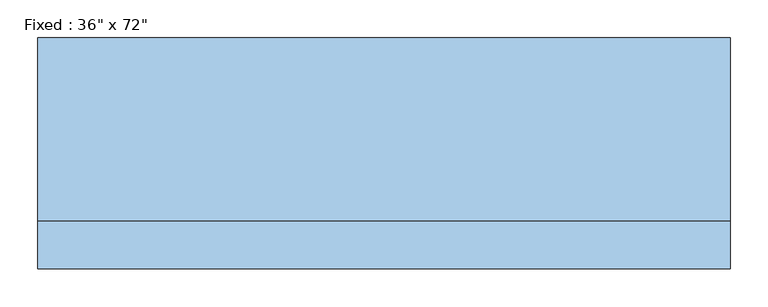
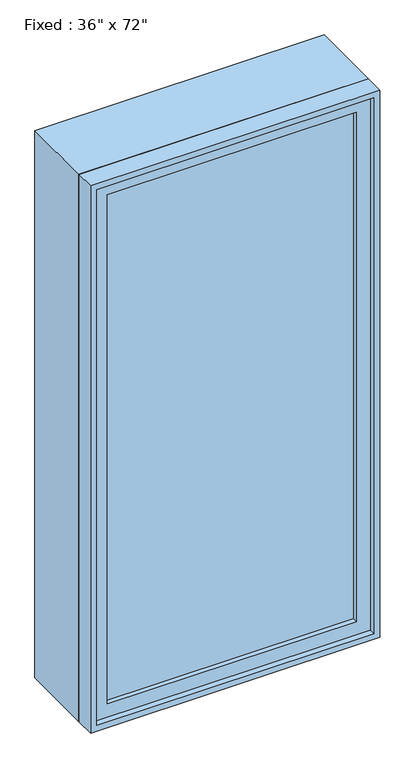
"""IFC4 building model written with IfcOpenShell, lengths in millimetres: window geometry."""

from ifc_helpers import new_model, si_unit, frame, origin, place, context, project, spatial, polyline, outline, extrude, source, transform, mapped, element, save


def window_9a1f8bc2(model_context):
    return source(origin(), model_context, "Body", "SweptSolid", [
        extrude(outline(polyline([(355.6, -104.775), (355.6, -117.475), (-431.8, -117.475), (-431.8, -104.775), (355.6, -104.775)])), frame((0.0, 0.0, 368.3), z_axis=(0.0, 0.0, 1.0), x_axis=(1.0, 0.0, 0.0)), (0.0, 0.0, 1.0), 1701.8),
        extrude(outline(polyline([(2114.55, -476.25), (323.85, -476.25), (323.85, 400.05), (2114.55, 400.05), (2114.55, -476.25)]), holes=[polyline([(2070.1, -431.8), (2070.1, 355.6), (368.3, 355.6), (368.3, -431.8), (2070.1, -431.8)])]), frame((0.0, -133.35, 0.0), z_axis=(0.0, 1.0, 0.0), x_axis=(0.0, 0.0, 1.0)), (0.0, 0.0, 1.0), 44.45),
        extrude(outline(polyline([(2133.6, -495.3), (304.8, -495.3), (304.8, 419.1), (2133.6, 419.1), (2133.6, -495.3)]), holes=[polyline([(2101.85, -463.55), (2101.85, 387.35), (336.55, 387.35), (336.55, -463.55), (2101.85, -463.55)])]), frame((0.0, -88.9, 0.0), z_axis=(0.0, 1.0, 0.0), x_axis=(0.0, 0.0, 1.0)), (0.0, 0.0, 1.0), 241.3),
        extrude(outline(polyline([(2133.6, 419.1), (2133.6, -495.3), (304.8, -495.3), (304.8, 419.1), (2133.6, 419.1)]), holes=[polyline([(2114.55, 400.05), (323.85, 400.05), (323.85, -476.25), (2114.55, -476.25), (2114.55, 400.05)])]), frame((0.0, -152.4, 0.0), z_axis=(0.0, 1.0, 0.0), x_axis=(0.0, 0.0, 1.0)), (0.0, 0.0, 1.0), 63.5),
    ])


if __name__ == "__main__":
    model = new_model("IFC4")
    model_context = context("Model", 3, world=origin())
    ifc_project = project(units=[si_unit("LENGTHUNIT", "METRE", prefix="MILLI")], contexts=[model_context])
    site = spatial("IfcSite", under=ifc_project)
    building = spatial("IfcBuilding", under=site)
    placement = place(None, origin())
    window_shape = window_9a1f8bc2(model_context)
    element("IfcWindow", 1, ObjectType="Fixed : 36\" x 72\"", at=placement, inside=building, context=model_context, shape_type="MappedRepresentation", body=[
        mapped(window_shape, transform((0.0, 0.0, 0.0), x_axis=(1.0, 0.0, 0.0), y_axis=(0.0, 1.0, 0.0), z_axis=(0.0, 0.0, 1.0))),
    ])
    save(model, "model.ifc")

# Revit data of these elements
# Type "Fixed : 36\" x 72\""
#   Type Mark = "9"
#   Construction Type Id = "GSP4R"
#   Assembly Code = "B2020100"
#   Analytic Construction = "1/8 in Pilkington single glazing"
#   Visual Light Transmittance = 0.9
#   Solar Heat Gain Coefficient = 0.78
#   Heat Transfer Coefficient (U) = 0.6496 BTU/(h·ft²·°F)
#   Height = 6' - 0"
#   Default Sill Height = 1' - 0"
#   Width = 3' - 0"
#   Window Inset = 0' - 0 3/4"
#   Define Thermal Properties by = 1
#   Glass Pane Material = Glass
#   Sash Material = Iron, Ductile
#   Wall Closure = (empty or 0)
# Element 1 (IfcWindow, "Fixed : 36\" x 72\"")
#   Materials on its faces: "Iron, Ductile", "Glass"
# Materials
#   "Glass": class "Glass", colour RGB 0 128 192, transparency 0.75, Description = "Soda Lime Glass", Cost = 0
#   "Iron, Ductile": class "Metal", colour RGB 0 0 0, transparency 0, Description = "Ductile cast iron", Cost = 0
